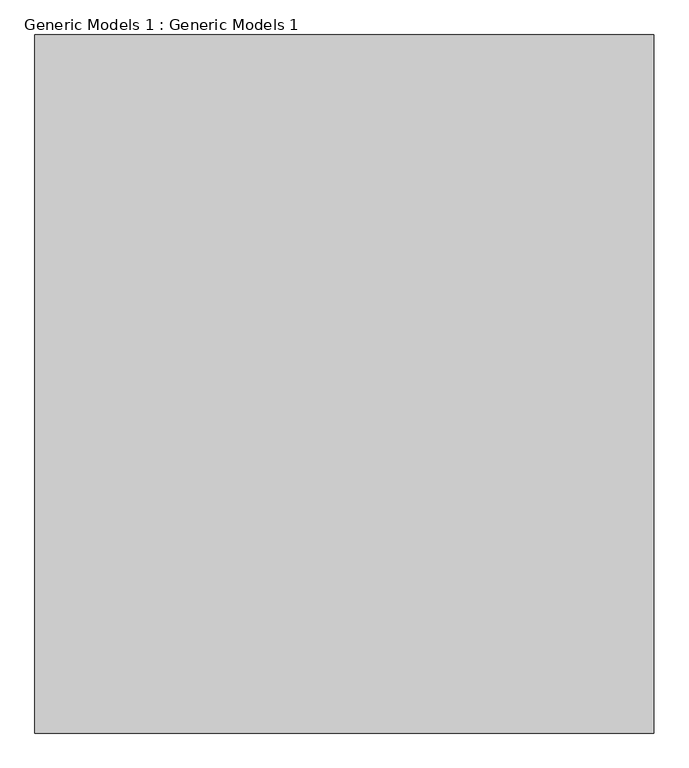
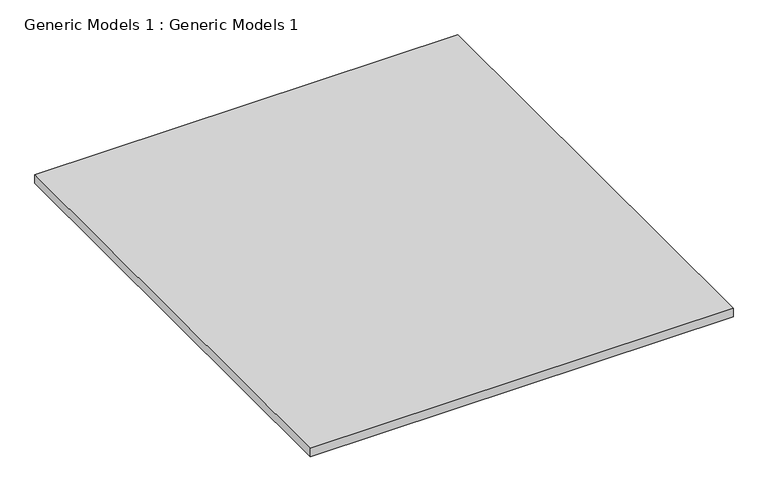
"""IFC4 building model written with IfcOpenShell, lengths in millimetres: proxy geometry, Generic Models 1 : Generic Models 1."""

from ifc_helpers import new_model, si_unit, frame, origin, place, context, project, spatial, polyline, outline, extrude, source, transform, mapped, element, save


def generic_models_1_generic_models_1_e43304c4(model_context):
    return source(origin(), model_context, "Body", "SweptSolid", [
        extrude(outline(polyline([(-6423.5125638, -0.5111724), (-6423.5125638, -16330.8026331), (-20900.9206529, -16330.8026331), (-20900.9206529, -0.5111724), (-6423.5125638, -0.5111724)])), frame((0.0, 0.0, -304.8), z_axis=(0.0, 0.0, 1.0), x_axis=(1.0, 0.0, 0.0)), (0.0, 0.0, 1.0), 304.8),
    ])


if __name__ == "__main__":
    model = new_model("IFC4")
    model_context = context("Model", 3, world=origin())
    ifc_project = project(units=[si_unit("LENGTHUNIT", "METRE", prefix="MILLI")], contexts=[model_context])
    site = spatial("IfcSite", under=ifc_project)
    building = spatial("IfcBuilding", under=site)
    placement = place(None, origin())
    generic_models_1_generic_models_1_shape = generic_models_1_generic_models_1_e43304c4(model_context)
    element("IfcBuildingElementProxy", 1, Name="Generic Models 1 : Generic Models 1", ObjectType="Generic Models 1 : Generic Models 1", at=placement, inside=building, context=model_context, shape_type="MappedRepresentation", body=[
        mapped(generic_models_1_generic_models_1_shape, transform((0.0, 0.0, 0.0), x_axis=(1.0, 0.0, 0.0), y_axis=(0.0, 1.0, 0.0), z_axis=(0.0, 0.0, 1.0))),
    ])
    save(model, "model.ifc")
